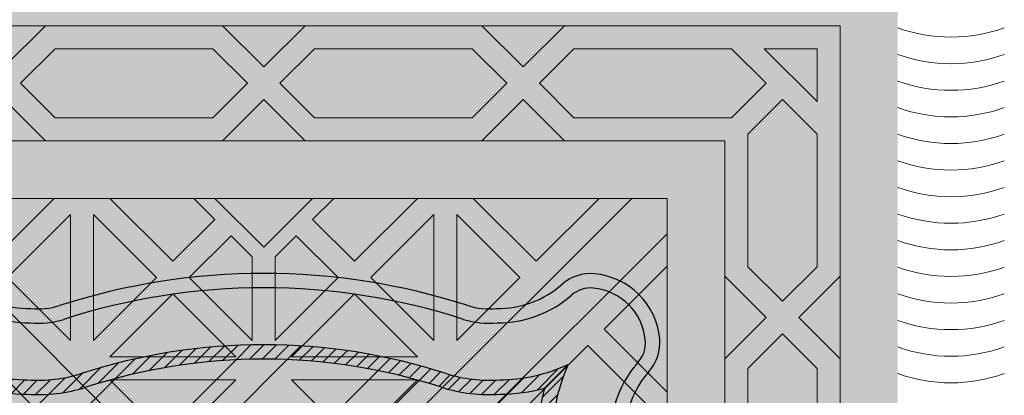
# Model space of a CAD drawing. Units: inches. Extents: x 844 to 2234, y 346 to 1084.
# Tile 62 of 93: x 1866.64 to 1877.53, y 708.75 to 712.91. Entities that reach past the tile are written whole.
import ezdxf

# ---------------------------------------------------------------- set-up
doc = ezdxf.new("R2010")
doc.units = ezdxf.units.IN
doc.header["$MEASUREMENT"] = 0
doc.layers.add('furniture', color=8, linetype='Continuous', lineweight=18)
doc.layers.add('RA-AP-01$0$INT', color=35, linetype='Continuous', lineweight=5)
doc.layers.add('RA-AP-01$0$FURN', color=3, linetype='Continuous')
doc.layers.add('RA-AP-01$0$WOOD', color=64, linetype='Continuous')

# ---------------------------------------------------------------- blocks, each defined once
blk = doc.blocks.new('A$C18D01794')
at = {"layer": 'RA-AP-01$0$INT'}
h = blk.add_hatch(color=256, dxfattribs=at)
h.paths.add_polyline_path([(4.35521, -6.15671), (4.35521, -8.05671), (5.45521, -8.05671), (5.45521, -6.15671)])
h.paths.add_polyline_path([(4.40521, -8.00671), (4.40521, -6.20671), (5.40521, -6.20671), (5.40521, -8.00671)], flags=16)
h = blk.add_hatch(color=256, dxfattribs=at)
h.paths.add_polyline_path([(4.50521, -7.5855), (4.46935, -7.54964), (4.50521, -7.51378), (4.50521, -7.38196), (4.46935, -7.34611), (4.50521, -7.31025), (4.50521, -7.17843), (4.46935, -7.14257), (4.50521, -7.10671), (4.47692, -7.10671), (4.45521, -7.12843), (4.43349, -7.10671), (4.40521, -7.10671), (4.44106, -7.14257), (4.40521, -7.17843), (4.40521, -7.31025), (4.44106, -7.34611), (4.40521, -7.38196), (4.40521, -7.51378), (4.44106, -7.54964), (4.40521, -7.5855), (4.40521, -7.71732), (4.44106, -7.75318), (4.40521, -7.78903), (4.40521, -8.00671), (4.64435, -8.00671), (4.68021, -7.97085), (4.71606, -8.00671), (4.86935, -8.00671), (4.90521, -7.97085), (4.94106, -8.00671), (5.09435, -8.00671), (5.13021, -7.97085), (5.16606, -8.00671), (5.40521, -8.00671), (5.40521, -7.78903), (5.36935, -7.75318), (5.40521, -7.71732), (5.40521, -7.5855), (5.36935, -7.54964), (5.40521, -7.51378), (5.40521, -7.38196), (5.36935, -7.34611), (5.40521, -7.31025), (5.40521, -7.17843), (5.36935, -7.14257), (5.40521, -7.10671), (5.37692, -7.10671), (5.35521, -7.12843), (5.33349, -7.10671), (5.30521, -7.10671), (5.34106, -7.14257), (5.30521, -7.17843), (5.30521, -7.31025), (5.34106, -7.34611), (5.30521, -7.38196), (5.30521, -7.51378), (5.34106, -7.54964), (5.30521, -7.5855), (5.30521, -7.71732), (5.34106, -7.75318), (5.30521, -7.78903), (5.30521, -7.90671), (5.16606, -7.90671), (5.13021, -7.94257), (5.09435, -7.90671), (4.94106, -7.90671), (4.90521, -7.94257), (4.86935, -7.90671), (4.71606, -7.90671), (4.68021, -7.94257), (4.64435, -7.90671), (4.50521, -7.90671), (4.50521, -7.78903), (4.46935, -7.75318), (4.50521, -7.71732)])
h.paths.add_polyline_path([(4.48521, -7.70903), (4.45521, -7.73903), (4.42521, -7.70903), (4.42521, -7.59378), (4.45521, -7.56378), (4.48521, -7.59378)], flags=16)
h.paths.add_polyline_path([(4.45521, -7.76732), (4.48521, -7.79732), (4.48521, -7.91257), (4.45521, -7.94257), (4.42521, -7.91257), (4.42521, -7.79732)], flags=16)
h.paths.add_polyline_path([(4.45521, -7.5355), (4.42521, -7.5055), (4.42521, -7.39025), (4.45521, -7.36025), (4.48521, -7.39025), (4.48521, -7.5055)], flags=16)
h.paths.add_polyline_path([(4.49935, -7.92671), (4.63606, -7.92671), (4.66606, -7.95671), (4.63606, -7.98671), (4.49935, -7.98671), (4.46935, -7.95671)], flags=16)
h.paths.add_polyline_path([(4.42521, -7.94085), (4.47106, -7.98671), (4.42521, -7.98671)], flags=16)
h.paths.add_polyline_path([(4.45521, -7.33196), (4.42521, -7.30196), (4.42521, -7.18671), (4.45521, -7.15671), (4.48521, -7.18671), (4.48521, -7.30196)], flags=16)
h.paths.add_polyline_path([(4.72435, -7.92671), (4.86106, -7.92671), (4.89106, -7.95671), (4.86106, -7.98671), (4.72435, -7.98671), (4.69435, -7.95671)], flags=16)
h.paths.add_polyline_path([(4.91935, -7.95671), (4.94935, -7.92671), (5.08606, -7.92671), (5.11606, -7.95671), (5.08606, -7.98671), (4.94935, -7.98671)], flags=16)
h.paths.add_polyline_path([(5.14435, -7.95671), (5.17435, -7.92671), (5.31106, -7.92671), (5.34106, -7.95671), (5.31106, -7.98671), (5.17435, -7.98671)], flags=16)
h.paths.add_polyline_path([(5.32521, -7.59378), (5.35521, -7.56378), (5.38521, -7.59378), (5.38521, -7.70903), (5.35521, -7.73903), (5.32521, -7.70903)], flags=16)
h.paths.add_polyline_path([(5.32521, -7.79732), (5.35521, -7.76732), (5.38521, -7.79732), (5.38521, -7.91257), (5.35521, -7.94257), (5.32521, -7.91257)], flags=16)
h.paths.add_polyline_path([(5.32521, -7.5055), (5.32521, -7.39025), (5.35521, -7.36025), (5.38521, -7.39025), (5.38521, -7.5055), (5.35521, -7.5355)], flags=16)
h.paths.add_polyline_path([(5.32521, -7.30196), (5.32521, -7.18671), (5.35521, -7.15671), (5.38521, -7.18671), (5.38521, -7.30196), (5.35521, -7.33196)], flags=16)
h.paths.add_polyline_path([(5.33935, -7.98671), (5.38521, -7.94085), (5.38521, -7.98671)], flags=16)
h = blk.add_hatch(color=256, dxfattribs=at)
h.paths.add_polyline_path([(4.46935, -7.14257), (4.50521, -7.17843), (4.50521, -7.10671)])
h.paths.add_polyline_path([(4.45521, -7.12843), (4.47692, -7.10671), (4.43349, -7.10671)])
h.paths.add_polyline_path([(4.40521, -7.17843), (4.44106, -7.14257), (4.40521, -7.10671)])
h.paths.add_polyline_path([(4.42521, -7.30196), (4.45521, -7.33196), (4.48521, -7.30196), (4.48521, -7.18671), (4.45521, -7.15671), (4.42521, -7.18671)])
h.paths.add_polyline_path([(4.50521, -7.38196), (4.50521, -7.31025), (4.46935, -7.34611)])
h.paths.add_polyline_path([(4.42521, -7.5055), (4.45521, -7.5355), (4.48521, -7.5055), (4.48521, -7.39025), (4.45521, -7.36025), (4.42521, -7.39025)])
h.paths.add_polyline_path([(4.42521, -7.70903), (4.45521, -7.73903), (4.48521, -7.70903), (4.48521, -7.59378), (4.45521, -7.56378), (4.42521, -7.59378)])
h.paths.add_polyline_path([(4.46935, -7.54964), (4.50521, -7.5855), (4.50521, -7.51378)])
h.paths.add_polyline_path([(4.40521, -7.5855), (4.44106, -7.54964), (4.40521, -7.51378)])
h.paths.add_polyline_path([(4.40521, -7.78903), (4.44106, -7.75318), (4.40521, -7.71732)])
h.paths.add_polyline_path([(4.46935, -7.75318), (4.50521, -7.78903), (4.50521, -7.71732)])
h.paths.add_polyline_path([(4.42521, -7.91257), (4.45521, -7.94257), (4.48521, -7.91257), (4.48521, -7.79732), (4.45521, -7.76732), (4.42521, -7.79732)])
h.paths.add_polyline_path([(4.42521, -7.98671), (4.47106, -7.98671), (4.42521, -7.94085)])
h.paths.add_polyline_path([(4.49935, -7.98671), (4.63606, -7.98671), (4.66606, -7.95671), (4.63606, -7.92671), (4.49935, -7.92671), (4.46935, -7.95671)])
h.paths.add_polyline_path([(4.68021, -7.94257), (4.71606, -7.90671), (4.64435, -7.90671)])
h.paths.add_polyline_path([(4.64435, -8.00671), (4.71606, -8.00671), (4.68021, -7.97085)])
h.paths.add_polyline_path([(4.72435, -7.98671), (4.86106, -7.98671), (4.89106, -7.95671), (4.86106, -7.92671), (4.72435, -7.92671), (4.69435, -7.95671)])
h.paths.add_polyline_path([(4.90521, -7.94257), (4.94106, -7.90671), (4.86935, -7.90671)])
h.paths.add_polyline_path([(4.86935, -8.00671), (4.94106, -8.00671), (4.90521, -7.97085)])
h.paths.add_polyline_path([(4.94935, -7.98671), (5.08606, -7.98671), (5.11606, -7.95671), (5.08606, -7.92671), (4.94935, -7.92671), (4.91935, -7.95671)])
h.paths.add_polyline_path([(5.13021, -7.94257), (5.16606, -7.90671), (5.09435, -7.90671)])
h.paths.add_polyline_path([(5.09435, -8.00671), (5.16606, -8.00671), (5.13021, -7.97085)])
h.paths.add_polyline_path([(5.17435, -7.98671), (5.31106, -7.98671), (5.34106, -7.95671), (5.31106, -7.92671), (5.17435, -7.92671), (5.14435, -7.95671)])
h.paths.add_polyline_path([(5.32521, -7.91257), (5.35521, -7.94257), (5.38521, -7.91257), (5.38521, -7.79732), (5.35521, -7.76732), (5.32521, -7.79732)])
h.paths.add_polyline_path([(5.33935, -7.98671), (5.38521, -7.98671), (5.38521, -7.94085)])
h.paths.add_polyline_path([(5.32521, -7.70903), (5.35521, -7.73903), (5.38521, -7.70903), (5.38521, -7.59378), (5.35521, -7.56378), (5.32521, -7.59378)])
h.paths.add_polyline_path([(5.30521, -7.78903), (5.34106, -7.75318), (5.30521, -7.71732)])
h.paths.add_polyline_path([(5.36935, -7.75318), (5.40521, -7.78903), (5.40521, -7.71732)])
h.paths.add_polyline_path([(5.40521, -7.5855), (5.40521, -7.51378), (5.36935, -7.54964)])
h.paths.add_polyline_path([(5.30521, -7.5855), (5.34106, -7.54964), (5.30521, -7.51378)])
h.paths.add_polyline_path([(5.32521, -7.5055), (5.35521, -7.5355), (5.38521, -7.5055), (5.38521, -7.39025), (5.35521, -7.36025), (5.32521, -7.39025)])
h.paths.add_polyline_path([(5.30521, -7.38196), (5.34106, -7.34611), (5.30521, -7.31025)])
h.paths.add_polyline_path([(5.32521, -7.30196), (5.35521, -7.33196), (5.38521, -7.30196), (5.38521, -7.18671), (5.35521, -7.15671), (5.32521, -7.18671)])
h.paths.add_polyline_path([(5.40458, -7.38134, -0.001218), (5.40521, -7.38111), (5.40521, -7.31025), (5.36935, -7.34611)])
h.paths.add_polyline_path([(5.36935, -7.14257), (5.40521, -7.17843), (5.40521, -7.10671)])
h.paths.add_polyline_path([(5.35521, -7.12843), (5.37692, -7.10671), (5.33349, -7.10671)])
h.paths.add_polyline_path([(5.30521, -7.17843), (5.34106, -7.14257), (5.30521, -7.10671)])
blk.add_hatch(color=256, dxfattribs=at).paths.add_polyline_path([(4.50521, -7.90671), (5.30521, -7.90671), (5.30521, -7.10671), (5.25521, -7.10671), (5.25521, -7.85671), (4.55521, -7.85671), (4.55521, -7.10671), (4.50521, -7.10671)])
h = blk.add_hatch(color=256, dxfattribs=at)
h.paths.add_polyline_path([(4.58592, -7.85671), (4.6142, -7.85671), (4.66885, -7.80207), (4.72349, -7.85671), (4.77177, -7.85671), (4.82642, -7.80207), (4.86278, -7.83843), (4.8445, -7.85671), (4.86278, -7.85671), (4.90521, -7.81429), (4.94763, -7.85671), (4.96592, -7.85671), (4.94763, -7.83843), (4.98399, -7.80207), (5.03864, -7.85671), (5.08692, -7.85671), (5.14157, -7.80207), (5.19621, -7.85671), (5.2245, -7.85671), (4.90521, -7.53742)])
h.paths.add_polyline_path([(4.89521, -7.57571), (4.89521, -7.685), (4.84056, -7.63035)], flags=16)
h.paths.add_polyline_path([(4.91521, -7.57571), (4.96985, -7.63035), (4.91521, -7.685)], flags=16)
h.paths.add_polyline_path([(4.82642, -7.64449), (4.88106, -7.69914), (4.77177, -7.69914)], flags=16)
h.paths.add_polyline_path([(4.98399, -7.64449), (5.03864, -7.69914), (4.92935, -7.69914)], flags=16)
h.paths.add_polyline_path([(4.88106, -7.71914), (4.82642, -7.77378), (4.77177, -7.71914)], flags=16)
h.paths.add_polyline_path([(4.92935, -7.71914), (5.03864, -7.71914), (4.98399, -7.77378)], flags=16)
h.paths.add_polyline_path([(4.89521, -7.73328), (4.89521, -7.806), (4.87692, -7.82429), (4.84056, -7.78793)], flags=16)
h.paths.add_polyline_path([(4.91521, -7.73328), (4.96985, -7.78793), (4.93349, -7.82429), (4.91521, -7.806)], flags=16)
h.paths.add_polyline_path([(4.75763, -7.73328), (4.81228, -7.78793), (4.75763, -7.84257)], flags=16)
h.paths.add_polyline_path([(4.73763, -7.73328), (4.73763, -7.84257), (4.68299, -7.78793)], flags=16)
h.paths.add_polyline_path([(5.05278, -7.73328), (5.05278, -7.84257), (4.99814, -7.78793)], flags=16)
h.paths.add_polyline_path([(5.07278, -7.73328), (5.12742, -7.78793), (5.07278, -7.84257)], flags=16)
h.paths.add_polyline_path([(4.93592, -7.50671), (5.25521, -7.826), (5.25521, -7.79772), (5.20056, -7.74307), (5.25521, -7.68843), (5.25521, -7.64014), (5.20056, -7.5855), (5.23692, -7.54914), (5.25521, -7.56742), (5.25521, -7.54914), (5.21278, -7.50671), (5.25521, -7.46429), (5.25521, -7.446), (5.23692, -7.46429), (5.20056, -7.42793), (5.25521, -7.37328), (5.25521, -7.325), (5.20056, -7.27035), (5.25521, -7.21571), (5.25521, -7.18742)])
h.paths.add_polyline_path([(5.04299, -7.42793), (5.09763, -7.37328), (5.09763, -7.48257)], flags=16)
h.paths.add_polyline_path([(5.02885, -7.44207), (5.08349, -7.49671), (4.9742, -7.49671)], flags=16)
h.paths.add_polyline_path([(5.11763, -7.37328), (5.17228, -7.42793), (5.11763, -7.48257)], flags=16)
h.paths.add_polyline_path([(5.08349, -7.51671), (5.02885, -7.57136), (4.9742, -7.51671)], flags=16)
h.paths.add_polyline_path([(5.13177, -7.35914), (5.18642, -7.41378), (5.24106, -7.35914)], flags=17)
h.paths.add_polyline_path([(5.13177, -7.49671), (5.18642, -7.44207), (5.22278, -7.47843), (5.2045, -7.49671)], flags=16)
h.paths.add_polyline_path([(5.09763, -7.53085), (5.09763, -7.64014), (5.04299, -7.5855)], flags=16)
h.paths.add_polyline_path([(5.13177, -7.33914), (5.24106, -7.33914), (5.18642, -7.28449)], flags=17)
h.paths.add_polyline_path([(5.13177, -7.51671), (5.2045, -7.51671), (5.22278, -7.535), (5.18642, -7.57136)], flags=16)
h.paths.add_polyline_path([(5.11763, -7.53085), (5.17228, -7.5855), (5.11763, -7.64014)], flags=16)
h.paths.add_polyline_path([(5.18642, -7.59964), (5.24106, -7.65429), (5.13177, -7.65429)], flags=16)
h.paths.add_polyline_path([(5.13177, -7.67429), (5.24106, -7.67429), (5.18642, -7.72893)], flags=16)
h.paths.add_polyline_path([(5.25521, -7.126), (5.25521, -7.10671), (4.55521, -7.10671), (4.55521, -7.126), (4.90521, -7.476)])
h.paths.add_polyline_path([(4.98399, -7.36893), (4.92935, -7.31429), (5.03864, -7.31429)], flags=16)
h.paths.add_polyline_path([(4.96985, -7.38307), (4.91521, -7.43772), (4.91521, -7.32843)], flags=16)
h.paths.add_polyline_path([(4.92935, -7.29429), (4.98399, -7.23964), (5.03864, -7.29429)], flags=16)
h.paths.add_polyline_path([(5.05278, -7.28014), (4.99814, -7.2255), (5.05278, -7.17085)], flags=16)
h.paths.add_polyline_path([(5.07278, -7.28014), (5.07278, -7.17085), (5.12742, -7.2255)], flags=16)
h.paths.add_polyline_path([(4.89521, -7.43772), (4.84056, -7.38307), (4.89521, -7.32843)], flags=16)
h.paths.add_polyline_path([(4.91521, -7.28014), (4.91521, -7.20742), (4.93349, -7.18914), (4.96985, -7.2255)], flags=16)
h.paths.add_polyline_path([(4.88106, -7.31429), (4.82642, -7.36893), (4.77177, -7.31429)], flags=16)
h.paths.add_polyline_path([(4.89521, -7.28014), (4.84056, -7.2255), (4.87692, -7.18914), (4.89521, -7.20742)], flags=16)
h.paths.add_polyline_path([(4.98399, -7.21136), (4.94763, -7.175), (4.96592, -7.15671), (5.03864, -7.15671)], flags=16)
h.paths.add_polyline_path([(4.88106, -7.29429), (4.77177, -7.29429), (4.82642, -7.23964)], flags=16)
h.paths.add_polyline_path([(4.90521, -7.19914), (4.86278, -7.15671), (4.94763, -7.15671)], flags=16)
h.paths.add_polyline_path([(5.14157, -7.21136), (5.08692, -7.15671), (5.19621, -7.15671)], flags=16)
h.paths.add_polyline_path([(4.82642, -7.21136), (4.77177, -7.15671), (4.8445, -7.15671), (4.86278, -7.175)], flags=16)
h.paths.add_polyline_path([(4.81228, -7.2255), (4.75763, -7.28014), (4.75763, -7.17085)], flags=16)
h.paths.add_polyline_path([(4.73763, -7.28014), (4.68299, -7.2255), (4.73763, -7.17085)], flags=16)
h.paths.add_polyline_path([(4.72349, -7.15671), (4.66885, -7.21136), (4.6142, -7.15671)], flags=16)
h.paths.add_polyline_path([(4.59763, -7.50671), (4.55521, -7.54914), (4.55521, -7.56742), (4.57349, -7.54914), (4.60985, -7.5855), (4.55521, -7.64014), (4.55521, -7.68843), (4.60985, -7.74307), (4.55521, -7.79772), (4.55521, -7.826), (4.8745, -7.50671), (4.55521, -7.18742), (4.55521, -7.21571), (4.60985, -7.27035), (4.55521, -7.325), (4.55521, -7.37328), (4.60985, -7.42793), (4.57349, -7.46429), (4.55521, -7.446), (4.55521, -7.46429)])
h.paths.add_polyline_path([(4.71278, -7.48257), (4.71278, -7.37328), (4.76742, -7.42793)], flags=16)
h.paths.add_polyline_path([(4.72692, -7.49671), (4.78157, -7.44207), (4.83621, -7.49671)], flags=16)
h.paths.add_polyline_path([(4.69278, -7.48257), (4.63814, -7.42793), (4.69278, -7.37328)], flags=16)
h.paths.add_polyline_path([(4.72692, -7.51671), (4.83621, -7.51671), (4.78157, -7.57136)], flags=16)
h.paths.add_polyline_path([(4.67864, -7.49671), (4.60592, -7.49671), (4.58763, -7.47843), (4.62399, -7.44207)], flags=16)
h.paths.add_polyline_path([(4.71278, -7.53085), (4.76742, -7.5855), (4.71278, -7.64014)], flags=16)
h.paths.add_polyline_path([(4.67864, -7.51671), (4.62399, -7.57136), (4.58763, -7.535), (4.60592, -7.51671)], flags=16)
h.paths.add_polyline_path([(4.69278, -7.53085), (4.69278, -7.64014), (4.63814, -7.5855)], flags=16)
h.paths.add_polyline_path([(4.62399, -7.41378), (4.67864, -7.35914), (4.56935, -7.35914)], flags=17)
h.paths.add_polyline_path([(4.62399, -7.59964), (4.67864, -7.65429), (4.56935, -7.65429)], flags=16)
h.paths.add_polyline_path([(4.67864, -7.33914), (4.62399, -7.28449), (4.56935, -7.33914)], flags=17)
h.paths.add_polyline_path([(4.67864, -7.67429), (4.62399, -7.72893), (4.56935, -7.67429)], flags=16)
h = blk.add_hatch(color=256, dxfattribs=at)
h.paths.add_polyline_path([(4.90521, -7.53742), (4.8745, -7.50671), (4.55521, -7.826), (4.55521, -7.85671), (4.58592, -7.85671)])
h.paths.add_polyline_path([(4.93592, -7.50671), (4.90521, -7.53742), (5.2245, -7.85671), (5.25521, -7.85671), (5.25521, -7.826)])
h.paths.add_polyline_path([(5.25521, -7.18742), (5.25521, -7.126), (4.90521, -7.476), (4.93592, -7.50671)])
h.paths.add_polyline_path([(4.8745, -7.50671), (4.90521, -7.476), (4.55521, -7.126), (4.55521, -7.18742)])
h = blk.add_hatch(color=256, dxfattribs=at)
h.paths.add_polyline_path([(5.02885, -7.57136), (4.9742, -7.51671), (5.08349, -7.51671)])
h.paths.add_polyline_path([(4.9742, -7.49671), (5.02885, -7.44207), (5.08349, -7.49671)])
h.paths.add_polyline_path([(5.04299, -7.42793), (5.09763, -7.37328), (5.09763, -7.48257)])
h.paths.add_polyline_path([(5.11763, -7.48257), (5.11763, -7.37328), (5.17228, -7.42793)])
h.paths.add_polyline_path([(5.13177, -7.49671), (5.18642, -7.44207), (5.22278, -7.47843), (5.2045, -7.49671)])
h.paths.add_polyline_path([(5.23692, -7.46429), (5.20056, -7.42793), (5.25521, -7.37328), (5.25521, -7.446)])
h.paths.add_polyline_path([(5.18642, -7.41378), (5.13177, -7.35914), (5.24106, -7.35914)])
h.paths.add_polyline_path([(5.13177, -7.33914), (5.18642, -7.28449), (5.24106, -7.33914)])
h.paths.add_polyline_path([(5.20056, -7.27035), (5.25521, -7.21571), (5.25521, -7.325)])
h.paths.add_polyline_path([(5.21278, -7.50671), (5.25521, -7.46429), (5.25521, -7.54914)])
h.paths.add_polyline_path([(5.13177, -7.51671), (5.2045, -7.51671), (5.22278, -7.535), (5.18642, -7.57136)])
h.paths.add_polyline_path([(5.11763, -7.64014), (5.11763, -7.53085), (5.17228, -7.5855)])
h.paths.add_polyline_path([(5.04299, -7.5855), (5.09763, -7.53085), (5.09763, -7.64014)])
h.paths.add_polyline_path([(5.13177, -7.65429), (5.18642, -7.59964), (5.24106, -7.65429)])
h.paths.add_polyline_path([(5.20056, -7.5855), (5.23692, -7.54914), (5.25521, -7.56742), (5.25521, -7.64014)])
h.paths.add_polyline_path([(5.18642, -7.72893), (5.13177, -7.67429), (5.24106, -7.67429)])
h.paths.add_polyline_path([(5.20056, -7.74307), (5.25521, -7.68843), (5.25521, -7.79772)])
h = blk.add_hatch(color=256, dxfattribs=at)
h.paths.add_polyline_path([(4.96985, -7.63035), (4.91521, -7.57571), (4.91521, -7.685)])
h.paths.add_polyline_path([(4.89521, -7.57571), (4.84056, -7.63035), (4.89521, -7.685)])
h.paths.add_polyline_path([(4.82642, -7.64449), (4.77177, -7.69914), (4.88106, -7.69914)])
h.paths.add_polyline_path([(4.88106, -7.71914), (4.77177, -7.71914), (4.82642, -7.77378)])
h.paths.add_polyline_path([(4.89521, -7.73328), (4.84056, -7.78793), (4.87692, -7.82429), (4.89521, -7.806)])
h.paths.add_polyline_path([(4.86278, -7.83843), (4.82642, -7.80207), (4.77177, -7.85671), (4.8445, -7.85671)])
h.paths.add_polyline_path([(4.81228, -7.78793), (4.75763, -7.73328), (4.75763, -7.84257)])
h.paths.add_polyline_path([(4.73763, -7.73328), (4.68299, -7.78793), (4.73763, -7.84257)])
h.paths.add_polyline_path([(4.66885, -7.80207), (4.6142, -7.85671), (4.72349, -7.85671)])
h.paths.add_polyline_path([(4.90521, -7.81429), (4.86278, -7.85671), (4.94763, -7.85671)])
h.paths.add_polyline_path([(4.91521, -7.73328), (4.91521, -7.806), (4.93349, -7.82429), (4.96985, -7.78793)])
h.paths.add_polyline_path([(5.03864, -7.71914), (4.92935, -7.71914), (4.98399, -7.77378)])
h.paths.add_polyline_path([(4.98399, -7.64449), (4.92935, -7.69914), (5.03864, -7.69914)])
h.paths.add_polyline_path([(5.05278, -7.73328), (4.99814, -7.78793), (5.05278, -7.84257)])
h.paths.add_polyline_path([(4.98399, -7.80207), (4.94763, -7.83843), (4.96592, -7.85671), (5.03864, -7.85671)])
h.paths.add_polyline_path([(5.12742, -7.78793), (5.07278, -7.73328), (5.07278, -7.84257)])
h.paths.add_polyline_path([(5.14157, -7.80207), (5.08692, -7.85671), (5.19621, -7.85671)])
for p, q in [((5.25521, -7.10671), (5.25521, -7.85671)), ((4.8745, -7.50671), (4.55521, -7.826)), ((4.93592, -7.50671), (5.25521, -7.826)), ((4.90521, -7.53742), (4.58592, -7.85671)), ((4.90521, -7.53742), (5.2245, -7.85671)), ((5.32521, -7.59378), (5.32521, -7.70903)), ((5.38521, -7.59378), (5.38521, -7.70903)), ((4.82642, -7.64449), (4.77177, -7.69914)), ((4.88106, -7.69914), (4.82642, -7.64449)), ((4.92935, -7.69914), (4.98399, -7.64449)), ((4.98399, -7.64449), (5.03864, -7.69914)), ((5.18642, -7.72893), (5.13177, -7.67429)), ((5.24106, -7.67429), (5.18642, -7.72893)), ((5.25521, -7.68843), (5.20056, -7.74307)), ((4.77177, -7.69914), (4.88106, -7.69914)), ((5.03864, -7.69914), (4.92935, -7.69914)), ((5.32521, -7.70903), (5.35521, -7.73903)), ((5.38521, -7.70903), (5.35521, -7.73903)), ((4.77177, -7.71914), (4.88106, -7.71914)), ((4.77177, -7.71914), (4.82642, -7.77378)), ((4.88106, -7.71914), (4.82642, -7.77378)), ((5.03864, -7.71914), (4.92935, -7.71914)), ((4.92935, -7.71914), (4.98399, -7.77378)), ((5.03864, -7.71914), (4.98399, -7.77378)), ((5.30521, -7.71732), (5.34106, -7.75318)), ((5.40521, -7.71732), (5.36935, -7.75318)), ((4.68299, -7.78793), (4.73763, -7.73328)), ((4.73763, -7.73328), (4.73763, -7.84257)), ((4.75763, -7.73328), (4.81228, -7.78793)), ((4.75763, -7.73328), (4.75763, -7.84257)), ((4.89521, -7.73328), (4.84056, -7.78793)), ((4.89521, -7.806), (4.89521, -7.73328)), ((4.91521, -7.806), (4.91521, -7.73328)), ((4.91521, -7.73328), (4.96985, -7.78793)), ((5.05278, -7.73328), (4.99814, -7.78793)), ((5.05278, -7.73328), (5.05278, -7.84257)), ((5.12742, -7.78793), (5.07278, -7.73328)), ((5.07278, -7.73328), (5.07278, -7.84257)), ((5.25521, -7.79772), (5.20056, -7.74307)), ((5.34106, -7.75318), (5.30521, -7.78903)), ((5.36935, -7.75318), (5.40521, -7.78903)), ((5.35521, -7.76732), (5.32521, -7.79732)), ((5.35521, -7.76732), (5.38521, -7.79732)), ((4.73763, -7.84257), (4.68299, -7.78793)), ((4.75763, -7.84257), (4.81228, -7.78793)), ((4.84056, -7.78793), (4.87692, -7.82429)), ((4.96985, -7.78793), (4.93349, -7.82429)), ((5.05278, -7.84257), (4.99814, -7.78793)), ((5.07278, -7.84257), (5.12742, -7.78793)), ((5.32521, -7.91257), (5.32521, -7.79732)), ((5.38521, -7.79732), (5.38521, -7.91257)), ((4.72349, -7.85671), (4.66885, -7.80207)), ((4.77177, -7.85671), (4.82642, -7.80207)), ((4.82642, -7.80207), (4.86278, -7.83843)), ((4.98399, -7.80207), (4.94763, -7.83843)), ((5.03864, -7.85671), (4.98399, -7.80207)), ((5.08692, -7.85671), (5.14157, -7.80207)), ((5.19621, -7.85671), (5.14157, -7.80207)), ((4.90521, -7.81429), (4.86278, -7.85671)), ((4.89521, -7.806), (4.87692, -7.82429)), ((4.90521, -7.81429), (4.94763, -7.85671)), ((4.91521, -7.806), (4.93349, -7.82429)), ((4.8445, -7.85671), (4.86278, -7.83843)), ((4.94763, -7.83843), (4.96592, -7.85671)), ((4.96592, -7.85671), (4.94763, -7.83843)), ((4.55521, -7.85671), (5.25521, -7.85671)), ((4.8445, -7.85671), (4.77177, -7.85671)), ((4.94763, -7.85671), (4.86278, -7.85671)), ((4.96592, -7.85671), (5.03864, -7.85671)), ((5.26721, -7.90671), (4.54321, -7.90671)), ((5.26721, -7.90671), (4.54321, -7.90671)), ((4.71606, -7.90671), (4.68021, -7.94257)), ((4.86935, -7.90671), (4.90521, -7.94257)), ((4.94106, -7.90671), (4.90521, -7.94257)), ((5.09435, -7.90671), (5.13021, -7.94257)), ((5.16606, -7.90671), (5.13021, -7.94257)), ((5.32521, -7.91257), (5.35521, -7.94257)), ((5.38521, -7.91257), (5.35521, -7.94257)), ((4.72435, -7.92671), (4.69435, -7.95671)), ((4.86106, -7.92671), (4.72435, -7.92671)), ((4.86106, -7.92671), (4.89106, -7.95671)), ((4.94935, -7.92671), (4.91935, -7.95671)), ((4.94935, -7.92671), (5.08606, -7.92671)), ((5.08606, -7.92671), (5.11606, -7.95671)), ((5.17435, -7.92671), (5.14435, -7.95671)), ((5.17435, -7.92671), (5.31106, -7.92671)), ((5.31106, -7.92671), (5.34106, -7.95671)), ((5.33935, -7.98671), (5.38521, -7.94085)), ((5.38521, -7.94085), (5.38521, -7.98671)), ((4.72435, -7.98671), (4.69435, -7.95671)), ((4.86106, -7.98671), (4.89106, -7.95671)), ((4.94935, -7.98671), (4.91935, -7.95671)), ((5.08606, -7.98671), (5.11606, -7.95671)), ((5.17435, -7.98671), (5.14435, -7.95671)), ((5.31106, -7.98671), (5.34106, -7.95671)), ((4.71606, -8.00671), (4.68021, -7.97085)), ((4.86935, -8.00671), (4.90521, -7.97085)), ((4.94106, -8.00671), (4.90521, -7.97085)), ((5.09435, -8.00671), (5.13021, -7.97085)), ((5.16606, -8.00671), (5.13021, -7.97085)), ((4.86106, -7.98671), (4.72435, -7.98671)), ((4.94935, -7.98671), (5.08606, -7.98671)), ((5.17435, -7.98671), (5.31106, -7.98671)), ((5.33935, -7.98671), (5.38521, -7.98671))]:
    blk.add_line(p, q, dxfattribs=at)
for points in [[(5.40521, -8.00671), (4.40521, -8.00671), (4.40521, -7.10671)], [(5.30521, -7.10671), (5.30521, -7.90671), (4.50521, -7.90671), (4.50521, -7.10671)], [(5.40521, -7.10671), (5.40521, -8.00671)]]:
    blk.add_lwpolyline(points, dxfattribs=at)
for centre in [(5.50141, -7.83286), (5.50141, -7.85596), (5.50141, -7.87906), (5.50141, -7.90216), (5.50141, -7.92526), (5.50141, -7.94836), (5.50141, -7.97146), (5.50141, -7.99456), (5.50141, -8.01766), (5.50141, -8.04076), (5.50141, -8.06386), (5.50141, -8.08696), (5.50141, -8.11006), (5.50141, -8.13316)]:
    blk.add_arc(centre, 0.13641, 70.20384, 109.79616, dxfattribs=at)
blk = doc.blocks.new('A$C32926AE1')
at = {"layer": 'RA-AP-01$0$WOOD'}
h = blk.add_hatch(color=256, dxfattribs=at)
h.dxf.hatch_style = 1
h.paths.add_polyline_path([(5.15743, 4.57348, -0.100949), (5.1554, 4.59337, -0.184266), (5.17225, 4.6388, 0.205661), (5.17956, 4.66132, 0.361434), (5.13435, 4.70652, 0.205661), (5.11183, 4.69921, -0.184266), (5.0664, 4.68237, -0.105531), (5.04566, 4.68467, 0.156764), (4.76389, 4.68467, -0.105531), (4.74314, 4.68237, -0.184266), (4.69771, 4.69921, 0.205661), (4.67519, 4.70652, 0.361434), (4.62998, 4.66132, 0.205661), (4.63729, 4.6388, -0.184266), (4.65414, 4.59337, -0.100949), (4.65211, 4.57348, 0.02141), (4.62975, 4.15671, 0.02141), (4.65211, 3.73994, -0.100949), (4.65414, 3.72006, -0.184266), (4.63729, 3.67463, 0.205661), (4.62998, 3.65211, 0.361434), (4.67519, 3.6069, 0.205661), (4.69771, 3.61421, -0.184266), (4.74314, 3.63106, -0.105531), (4.76389, 3.62875, 0.156764), (5.04566, 3.62875, -0.105531), (5.0664, 3.63106, -0.184266), (5.11183, 3.61421, 0.205661), (5.13435, 3.6069, 0.361434), (5.17956, 3.65211, 0.205661), (5.17225, 3.67463, -0.184266), (5.1554, 3.72006, -0.100949), (5.15743, 3.73994, 0.02141), (5.17979, 4.15671, 0.02141)])
h.paths.add_polyline_path([(4.63975, 4.15671, 0.021354), (4.66197, 3.74189, -0.094076), (4.66414, 3.71961, -0.182482), (4.64481, 3.66804, 0.205661), (4.63994, 3.65302, 0.361434), (4.67611, 3.61686, 0.205661), (4.69112, 3.62173, -0.182482), (4.7427, 3.64106, -0.102989), (4.76699, 3.63826, 0.156709), (5.04255, 3.63826, -0.102989), (5.06685, 3.64106, -0.182482), (5.11842, 3.62173, 0.205661), (5.13344, 3.61686, 0.361434), (5.1696, 3.65302, 0.205661), (5.16473, 3.66804, -0.182482), (5.1454, 3.71961, -0.094076), (5.14757, 3.74189, 0.021354), (5.16979, 4.15671, 0.021354), (5.14757, 4.57154, -0.094076), (5.1454, 4.59381, -0.182482), (5.16473, 4.64539, 0.205661), (5.1696, 4.6604, 0.361434), (5.13344, 4.69657, 0.205661), (5.11842, 4.69169, -0.182482), (5.06685, 4.67236, -0.102989), (5.04255, 4.67517, 0.156709), (4.76699, 4.67517, -0.102989), (4.7427, 4.67236, -0.182482), (4.69112, 4.69169, 0.205661), (4.67611, 4.69657, 0.361434), (4.63994, 4.6604, 0.205661), (4.64481, 4.64539, -0.182482), (4.66414, 4.59381, -0.094076), (4.66197, 4.57154, 0.021354)], flags=16)
h.paths.add_polyline_path([(5.12979, 4.43217, -0.014166), (5.13015, 4.15693, -0.014166), (5.12979, 3.88169, -0.078525), (5.1098, 3.75514, 0.094597), (5.10541, 3.7179, 0.104317), (5.11607, 3.67039, 0.104317), (5.06856, 3.68105, 0.094597), (5.03132, 3.67666, -0.158024), (4.77823, 3.67666, 0.094597), (4.74098, 3.68105, 0.104317), (4.69347, 3.67039, 0.104317), (4.70413, 3.7179, 0.094597), (4.69975, 3.75514, -0.078525), (4.67975, 3.88169, -0.014166), (4.67939, 4.15693, -0.014166), (4.67975, 4.43217, -0.078525), (4.69975, 4.55871, 0.094597), (4.70413, 4.59596, 0.104317), (4.69347, 4.64347, 0.104317), (4.74098, 4.6328, 0.094597), (4.77823, 4.63719, -0.158024), (5.03132, 4.63719, 0.094597), (5.06856, 4.6328, 0.104317), (5.11607, 4.64347, 0.104317), (5.10541, 4.59596, 0.094597), (5.1098, 4.55871, -0.078525)], flags=0)
h.paths.add_polyline_path([(5.11979, 4.43226, -0.0142), (5.12016, 4.15693, -0.0142), (5.11979, 3.8816, -0.078489), (5.10027, 3.75819, 0.094014), (5.09541, 3.71748, 0.060627), (5.09962, 3.68684, 0.060627), (5.06898, 3.69105, 0.094014), (5.02827, 3.68619, -0.158071), (4.78127, 3.68619, 0.094014), (4.74056, 3.69105, 0.060627), (4.70993, 3.68684, 0.060627), (4.71413, 3.71748, 0.094014), (4.70927, 3.75819, -0.078489), (4.68975, 3.8816, -0.0142), (4.68939, 4.15693, -0.0142), (4.68975, 4.43226, -0.078489), (4.70927, 4.55566, 0.094014), (4.71413, 4.59638, 0.060627), (4.70993, 4.62701, 0.060627), (4.74056, 4.62281, 0.094014), (4.78127, 4.62767, -0.158071), (5.02827, 4.62767, 0.094014), (5.06898, 4.62281, 0.060627), (5.09962, 4.62701, 0.060627), (5.09541, 4.59638, 0.094014), (5.10027, 4.55566, -0.078489)], flags=0)
h.paths.add_polyline_path([(5.06979, 4.43022, -0.014242), (5.07017, 4.15693, -0.014242), (5.06979, 3.88364, -0.080061), (5.05266, 3.77346, 0.052642), (5.04591, 3.74055, 0.052642), (5.013, 3.7338, -0.158303), (4.79655, 3.7338, 0.052642), (4.76363, 3.74055, 0.052642), (4.75688, 3.77346, -0.080061), (4.73975, 3.88364, -0.014242), (4.73937, 4.15693, -0.014242), (4.73975, 4.43022, -0.080061), (4.75688, 4.54039, 0.052642), (4.76363, 4.5733, 0.052642), (4.79655, 4.58006, -0.158303), (5.013, 4.58006, 0.052642), (5.04591, 4.5733, 0.052642), (5.05266, 4.54039, -0.080061)], flags=0)
h.paths.add_polyline_path([(5.04979, 4.43038, -0.01431), (5.05018, 4.15693, -0.01431), (5.04979, 3.88347, -0.080069), (5.03362, 3.77958, 0.030626), (5.02824, 3.75822, 0.030626), (5.00688, 3.75284, -0.158398), (4.80266, 3.75284, 0.030626), (4.7813, 3.75822, 0.030626), (4.77592, 3.77958, -0.080069), (4.75975, 3.88347, -0.01431), (4.75936, 4.15693, -0.01431), (4.75975, 4.43038, -0.080069), (4.77592, 4.53427, 0.030626), (4.7813, 4.55564, 0.030626), (4.80266, 4.56102, -0.158398), (5.00688, 4.56102, 0.030626), (5.02824, 4.55564, 0.030626), (5.03362, 4.53427, -0.080069)], flags=0)
h.paths.add_polyline_path([(4.99977, 4.42817, -0.014344), (5.0002, 4.15693, -0.014344), (4.99977, 3.88568, -0.078464), (4.98736, 3.7991, -0.150605), (4.82219, 3.7991, -0.078464), (4.80978, 3.88568, -0.014344), (4.80934, 4.15693, -0.014344), (4.80978, 4.42817, -0.078464), (4.82219, 4.51475, -0.150605), (4.98736, 4.51475, -0.078464)], flags=0)
h.paths.add_polyline_path([(4.97976, 4.42764, -0.014377), (4.98021, 4.15693, -0.014377), (4.97976, 3.88621, -0.068924), (4.97118, 3.81528, -0.129665), (4.83836, 3.81528, -0.068924), (4.82979, 3.88621, -0.014377), (4.82934, 4.15693, -0.014377), (4.82979, 4.42764, -0.068924), (4.83836, 4.49858, -0.129665), (4.97118, 4.49858, -0.068924)], flags=0)
h = blk.add_hatch(color=256, dxfattribs=at)
h.dxf.hatch_style = 1
h.paths.add_polyline_path([(5.1454, 4.59381, -0.182482), (5.16473, 4.64539, 0.205661), (5.1696, 4.6604, 0.361434), (5.13344, 4.69657, 0.205661), (5.11842, 4.69169, -0.182482), (5.06685, 4.67236, -0.102989), (5.04255, 4.67517, 0.156709), (4.76699, 4.67517, -0.102989), (4.7427, 4.67236, -0.182482), (4.69112, 4.69169, 0.205661), (4.67611, 4.69657, 0.361434), (4.63994, 4.6604, 0.205661), (4.64481, 4.64539, -0.182482), (4.66414, 4.59381, -0.094076), (4.66197, 4.57154, 0.021354), (4.63975, 4.15671, 0.021354), (4.66197, 3.74189, -0.094076), (4.66414, 3.71961, -0.182482), (4.64481, 3.66804, 0.205661), (4.63994, 3.65302, 0.361434), (4.67611, 3.61686, 0.205661), (4.69112, 3.62173, -0.182482), (4.7427, 3.64106, -0.102989), (4.76699, 3.63826, 0.156709), (5.04255, 3.63826, -0.102989), (5.06685, 3.64106, -0.182482), (5.11842, 3.62173, 0.205661), (5.13344, 3.61686, 0.361434), (5.1696, 3.65302, 0.205661), (5.16473, 3.66804, -0.182482), (5.1454, 3.71961, -0.094076), (5.14757, 3.74189, 0.021354), (5.16979, 4.15671, 0.021354), (5.14757, 4.57154, -0.094076)])
h.paths.add_polyline_path([(5.1098, 4.55871, -0.078525), (5.12979, 4.43217, -0.014166), (5.13015, 4.15693, -0.014166), (5.12979, 3.88169, -0.078525), (5.1098, 3.75514, 0.094597), (5.10541, 3.7179, 0.104317), (5.11607, 3.67039, 0.104317), (5.06856, 3.68105, 0.094597), (5.03132, 3.67666, -0.158024), (4.77823, 3.67666, 0.094597), (4.74098, 3.68105, 0.104317), (4.69347, 3.67039, 0.104317), (4.70413, 3.7179, 0.094597), (4.69975, 3.75514, -0.078525), (4.67975, 3.88169, -0.014166), (4.67939, 4.15693, -0.014166), (4.67975, 4.43217, -0.078525), (4.69975, 4.55871, 0.094597), (4.70413, 4.59596, 0.104317), (4.69347, 4.64347, 0.104317), (4.74098, 4.6328, 0.094597), (4.77823, 4.63719, -0.158024), (5.03132, 4.63719, 0.094597), (5.06856, 4.6328, 0.104317), (5.11607, 4.64347, 0.104317), (5.10541, 4.59596, 0.094597)], flags=16)
h.paths.add_polyline_path([(5.10027, 4.55566, -0.078489), (5.11979, 4.43226, -0.0142), (5.12016, 4.15693, -0.0142), (5.11979, 3.8816, -0.078489), (5.10027, 3.75819, 0.094014), (5.09541, 3.71748, 0.060627), (5.09962, 3.68684, 0.060627), (5.06898, 3.69105, 0.094014), (5.02827, 3.68619, -0.158071), (4.78127, 3.68619, 0.094014), (4.74056, 3.69105, 0.060627), (4.70993, 3.68684, 0.060627), (4.71413, 3.71748, 0.094014), (4.70927, 3.75819, -0.078489), (4.68975, 3.8816, -0.0142), (4.68939, 4.15693, -0.0142), (4.68975, 4.43226, -0.078489), (4.70927, 4.55566, 0.094014), (4.71413, 4.59638, 0.060627), (4.70993, 4.62701, 0.060627), (4.74056, 4.62281, 0.094014), (4.78127, 4.62767, -0.158071), (5.02827, 4.62767, 0.094014), (5.06898, 4.62281, 0.060627), (5.09962, 4.62701, 0.060627), (5.09541, 4.59638, 0.094014)], flags=0)
h.paths.add_polyline_path([(5.04591, 4.5733, 0.052642), (5.05266, 4.54039, -0.080061), (5.06979, 4.43022, -0.014242), (5.07017, 4.15693, -0.014242), (5.06979, 3.88364, -0.080061), (5.05266, 3.77346, 0.052642), (5.04591, 3.74055, 0.052642), (5.013, 3.7338, -0.158303), (4.79655, 3.7338, 0.052642), (4.76363, 3.74055, 0.052642), (4.75688, 3.77346, -0.080061), (4.73975, 3.88364, -0.014242), (4.73937, 4.15693, -0.014242), (4.73975, 4.43022, -0.080061), (4.75688, 4.54039, 0.052642), (4.76363, 4.5733, 0.052642), (4.79655, 4.58006, -0.158303), (5.013, 4.58006, 0.052642)], flags=0)
h.paths.add_polyline_path([(5.02824, 4.55564, 0.030626), (5.03362, 4.53427, -0.080069), (5.04979, 4.43038, -0.01431), (5.05018, 4.15693, -0.01431), (5.04979, 3.88347, -0.080069), (5.03362, 3.77958, 0.030626), (5.02824, 3.75822, 0.030626), (5.00688, 3.75284, -0.158398), (4.80266, 3.75284, 0.030626), (4.7813, 3.75822, 0.030626), (4.77592, 3.77958, -0.080069), (4.75975, 3.88347, -0.01431), (4.75936, 4.15693, -0.01431), (4.75975, 4.43038, -0.080069), (4.77592, 4.53427, 0.030626), (4.7813, 4.55564, 0.030626), (4.80266, 4.56102, -0.158398), (5.00688, 4.56102, 0.030626)], flags=0)
h.paths.add_polyline_path([(4.98736, 4.51475, -0.078464), (4.99977, 4.42817, -0.014344), (5.0002, 4.15693, -0.014344), (4.99977, 3.88568, -0.078464), (4.98736, 3.7991, -0.150605), (4.82219, 3.7991, -0.078464), (4.80978, 3.88568, -0.014344), (4.80934, 4.15693, -0.014344), (4.80978, 4.42817, -0.078464), (4.82219, 4.51475, -0.150605)], flags=0)
h.paths.add_polyline_path([(4.97118, 4.49858, -0.068924), (4.97976, 4.42764, -0.014377), (4.98021, 4.15693, -0.014377), (4.97976, 3.88621, -0.068924), (4.97118, 3.81528, -0.129665), (4.83836, 3.81528, -0.068924), (4.82979, 3.88621, -0.014377), (4.82934, 4.15693, -0.014377), (4.82979, 4.42764, -0.068924), (4.83836, 4.49858, -0.129665)], flags=0)
h = blk.add_hatch(dxfattribs=at)
h.set_pattern_fill('ANSI31', color=256, scale=0.05, style=0)
h.paths.add_polyline_path([(5.13015, 4.15693, 0.014166), (5.12979, 4.43217, 0.077783), (5.11017, 4.55756, -0.097652), (5.10541, 4.59596, -0.104317), (5.11607, 4.64347), (5.09962, 4.62701, 0.060627), (5.09541, 4.59638, 0.094014), (5.10027, 4.55566, -0.078489), (5.11979, 4.43226, -0.0142), (5.12016, 4.15693, -0.0142), (5.11979, 3.8816, -0.078489), (5.10027, 3.75819, 0.094014), (5.09541, 3.71748, 0.060627), (5.09962, 3.68684), (5.11607, 3.67039, -0.104317), (5.10541, 3.7179, -0.097652), (5.11017, 3.7563, 0.077783), (5.12979, 3.88169, 0.014166)])
h.paths.add_polyline_path([(5.03016, 3.67629, -0.097652), (5.06856, 3.68105, -0.104317), (5.11607, 3.67039), (5.09962, 3.68684, 0.060627), (5.06898, 3.69105, 0.094014), (5.02827, 3.68619, -0.158071), (4.78127, 3.68619, 0.094014), (4.74056, 3.69105, 0.060627), (4.70993, 3.68684), (4.69347, 3.67039, -0.104317), (4.74098, 3.68105, -0.097652), (4.77938, 3.67629, 0.156513)])
h.paths.add_polyline_path([(4.68975, 3.8816, -0.0142), (4.68939, 4.15693, -0.0142), (4.68975, 4.43226, -0.078489), (4.70927, 4.55566, 0.094014), (4.71413, 4.59638, 0.060627), (4.70993, 4.62701), (4.69347, 4.64347, -0.104317), (4.70413, 4.59596, -0.097652), (4.69937, 4.55756, 0.077783), (4.67975, 4.43217, 0.014166), (4.67939, 4.15693, 0.014166), (4.67975, 3.88169, 0.077783), (4.69937, 3.7563, -0.097652), (4.70413, 3.7179, -0.104317), (4.69347, 3.67039), (4.70993, 3.68684, 0.060627), (4.71413, 3.71748, 0.094014), (4.70927, 3.75819, -0.078489)])
h.paths.add_polyline_path([(4.77938, 4.63756, -0.097652), (4.74098, 4.6328, -0.104317), (4.69347, 4.64347), (4.70993, 4.62701, 0.060627), (4.74056, 4.62281, 0.094014), (4.78127, 4.62767, -0.158071), (5.02827, 4.62767, 0.094014), (5.06898, 4.62281, 0.060627), (5.09962, 4.62701), (5.11607, 4.64347, -0.104317), (5.06856, 4.6328, -0.097652), (5.03016, 4.63756, 0.156513)])
h = blk.add_hatch(dxfattribs=at)
h.set_pattern_fill('ANSI32', color=256, scale=0.2, style=0)
h.paths.add_polyline_path([(5.11979, 4.43226, 0.077702), (5.10066, 4.55447, -0.09689), (5.09541, 4.59638, -0.060627), (5.09962, 4.62701, -0.060627), (5.06898, 4.62281, -0.09689), (5.02707, 4.62805, 0.156466), (4.78247, 4.62805, -0.09689), (4.74056, 4.62281, -0.060627), (4.70993, 4.62701, -0.060627), (4.71413, 4.59638, -0.09689), (4.70888, 4.55447, 0.077702), (4.68975, 4.43226, 0.0142), (4.68939, 4.15693, 0.0142), (4.68975, 3.8816, 0.077702), (4.70888, 3.75939, -0.09689), (4.71413, 3.71748, -0.060627), (4.70993, 3.68684, -0.060627), (4.74056, 3.69105, -0.09689), (4.78247, 3.6858, 0.156466), (5.02707, 3.6858, -0.09689), (5.06898, 3.69105, -0.060627), (5.09962, 3.68684, -0.060627), (5.09541, 3.71748, -0.09689), (5.10066, 3.75939, 0.077702), (5.11979, 3.8816, 0.0142), (5.12016, 4.15693, 0.0142)])
h.paths.add_polyline_path([(5.07017, 4.15693, -0.014242), (5.06979, 3.88364, -0.080061), (5.05266, 3.77346, 0.052642), (5.04591, 3.74055, 0.052642), (5.013, 3.7338, -0.158303), (4.79655, 3.7338, 0.052642), (4.76363, 3.74055, 0.052642), (4.75688, 3.77346, -0.080061), (4.73975, 3.88364, -0.014242), (4.73937, 4.15693, -0.014242), (4.73975, 4.43022, -0.080061), (4.75688, 4.54039, 0.052642), (4.76363, 4.5733, 0.052642), (4.79655, 4.58006, -0.158303), (5.013, 4.58006, 0.052642), (5.04591, 4.5733, 0.052642), (5.05266, 4.54039, -0.080061), (5.06979, 4.43022, -0.014242)], flags=16)
h.paths.add_polyline_path([(5.05018, 4.15693, -0.01431), (5.04979, 3.88347, -0.080069), (5.03362, 3.77958, 0.030626), (5.02824, 3.75822, 0.030626), (5.00688, 3.75284, -0.158398), (4.80266, 3.75284, 0.030626), (4.7813, 3.75822, 0.030626), (4.77592, 3.77958, -0.080069), (4.75975, 3.88347, -0.01431), (4.75936, 4.15693, -0.01431), (4.75975, 4.43038, -0.080069), (4.77592, 4.53427, 0.030626), (4.7813, 4.55564, 0.030626), (4.80266, 4.56102, -0.158398), (5.00688, 4.56102, 0.030626), (5.02824, 4.55564, 0.030626), (5.03362, 4.53427, -0.080069), (5.04979, 4.43038, -0.01431)], flags=0)
h.paths.add_polyline_path([(5.0002, 4.15693, -0.014344), (4.99977, 3.88568, -0.078464), (4.98736, 3.7991, -0.150605), (4.82219, 3.7991, -0.078464), (4.80978, 3.88568, -0.014344), (4.80934, 4.15693, -0.014344), (4.80978, 4.42817, -0.078464), (4.82219, 4.51475, -0.150605), (4.98736, 4.51475, -0.078464), (4.99977, 4.42817, -0.014344)], flags=0)
h.paths.add_polyline_path([(4.98021, 4.15693, -0.014377), (4.97976, 3.88621, -0.068924), (4.97118, 3.81528, -0.129665), (4.83836, 3.81528, -0.068924), (4.82979, 3.88621, -0.014377), (4.82934, 4.15693, -0.014377), (4.82979, 4.42764, -0.068924), (4.83836, 4.49858, -0.129665), (4.97118, 4.49858, -0.068924), (4.97976, 4.42764, -0.014377)], flags=0)
blk.add_line((5.09962, 4.62701), (5.11607, 4.64347), dxfattribs=at)
blk.add_line((5.09962, 4.62701), (5.11607, 4.64347), dxfattribs=at)
for centre, radius, start, end in [((4.90477, 4.24636), 0.4604, 72.06839, 107.93161), ((5.1316, 4.67665), 0.03, 84.74312, 131.22895), ((5.12977, 4.65674), 0.05, 5.25688, 84.74312), ((4.74251, 4.75033), 0.06797, 228.77105, 270.53331), ((4.90477, 4.24636), 0.4504, 72.06232, 107.93768), ((5.06703, 4.75033), 0.06797, 269.46669, 311.22895), ((5.1316, 4.67665), 0.02, 84.74312, 131.22895), ((5.12977, 4.65674), 0.04, 5.25688, 84.74312), ((4.74251, 4.75033), 0.07797, 228.77105, 270.13765), ((5.06703, 4.75033), 0.07797, 269.86235, 311.22895), ((4.74811, 4.73212), 0.05, 264.29793, 287.35568), ((5.06143, 4.73212), 0.05, 252.64432, 275.70207), ((4.74811, 4.73212), 0.06, 264.82381, 287.40613), ((5.06143, 4.73212), 0.06, 252.59387, 275.17619), ((5.14969, 4.65857), 0.02, 318.77105, 5.25688), ((5.14969, 4.65857), 0.03, 318.77105, 5.25688), ((4.90477, 4.24679), 0.4104, 72.0403, 107.9597), ((4.90477, 4.24679), 0.4004, 72.03508, 107.96492), ((4.74251, 4.75076), 0.11797, 245.43667, 269.25822), ((5.06703, 4.75076), 0.11797, 270.74178, 294.56333), ((5.22337, 4.59443), 0.11797, 155.43667, 179.25822), ((5.22337, 4.594), 0.07797, 138.77105, 180.13765), ((4.74811, 4.73255), 0.1, 265.91267, 287.52837), ((5.06143, 4.73255), 0.1, 252.47163, 274.08733), ((5.22337, 4.594), 0.06797, 138.77105, 180.53331), ((4.74251, 4.75076), 0.12797, 255.25019, 269.12793), ((4.74811, 4.73255), 0.11, 266.06531, 287.54856), ((5.06143, 4.73255), 0.11, 252.45144, 273.93469), ((5.06703, 4.75076), 0.12797, 270.87207, 284.74981), ((5.22337, 4.59443), 0.12797, 165.25019, 179.12793)]:
    blk.add_arc(centre, radius, start, end, dxfattribs=at)
blk = doc.blocks.new('A$C5D2F253E')
at = {"layer": 'RA-AP-01$0$FURN', "xscale": -0.7999999999883585, "yscale": 0.7999999999883585, "zscale": 0.8, "rotation": 90}
blk.add_blockref('A$C18D01794', (-5.68776, 4.75792), dxfattribs=at)
at = {"layer": 'RA-AP-01$0$WOOD', "rotation": 270}
blk.add_blockref('A$C32926AE1', (-4.16134, 5.73853), dxfattribs=at)

msp = doc.modelspace()

# ---------------------------------------------------------------- block references
at = {"layer": 'furniture', "xscale": 15.94108302203742, "yscale": 15.94108302203742, "zscale": 15.94108302203742, "rotation": 90}
msp.add_blockref('A$C5D2F253E', (1882.631, 701.403), dxfattribs=at)

doc.saveas('drawing.dxf')
